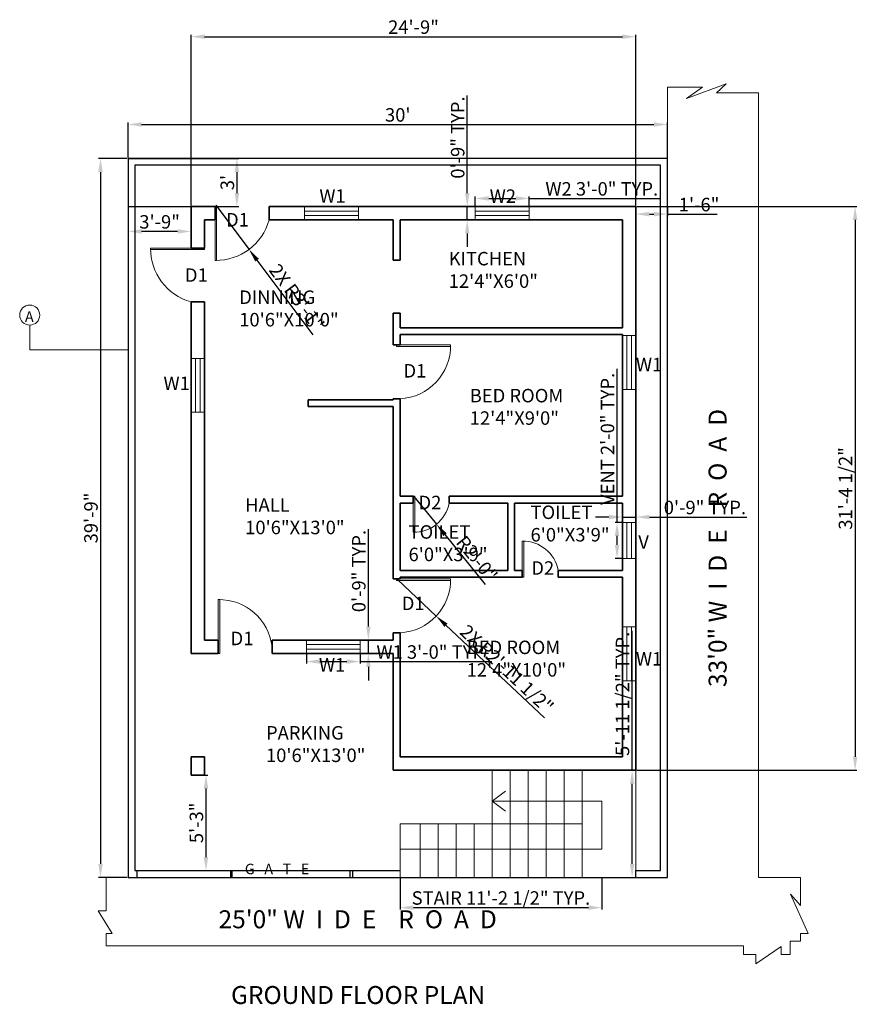
# Model space of a CAD drawing. Units: inches. Extents: x 2044 to 3644, y 808 to 1988.
# Tile 1 of 4: x 2044 to 2610, y 808 to 1466. Entities that reach past the tile are written whole.
import ezdxf

# ---------------------------------------------------------------- set-up
doc = ezdxf.new("R2010")
doc.units = ezdxf.units.IN
for name, color, linetype, lineweight in [('A-ANNO-DIMS', 2, 'Continuous', 18), ('A-ANNO-SYMB', 2, 'Continuous', 18), ('A-ANNO-TEXT', 7, 'Continuous', 18), ('A-ANNO-TITL', 7, 'Continuous', 25), ('A-AREA-IDEN', 7, 'Continuous', 18), ('A-COLS', 1, 'Continuous', 35), ('A-DOOR', 4, 'Continuous', 18), ('A-FLOR-STRS', 3, 'Continuous', 18), ('A-GLAZ', 4, 'Continuous', 18), ('A-WALL', 7, 'Continuous', 35), ('C-PROP', 3, 'Continuous', 25), ('C-ROAD', 8, 'Continuous', 18)]:
    doc.layers.add(name, color=color, linetype=linetype, lineweight=lineweight)
doc.styles.get("Standard").update_dxf_attribs({"font": 'arial.ttf'})
doc.dimstyles.new('ISO-25', dxfattribs={"dimtxt": 9, "dimasz": 9, "dimexe": 1.25, "dimexo": 0.625, "dimtad": 1, "dimdec": 1, "dimrnd": 9, "dimlunit": 3, "dimtxsty": 'Standard', "dimcen": 2.5, "dimadec": 0, "dimazin": 0, "dimtfac": 1, "dimtdec": 1, "dimtmove": 0, "dimatfit": 3, "dimfxl": 1, "dimarcsym": 0})

# ---------------------------------------------------------------- blocks, each defined once
blk = doc.blocks.new('*D1')
at = {"layer": 'A-ANNO-DIMS', "color": 0, "lineweight": -2, "transparency": 16777216}
for p, q in [((2455.33, 1340.62), (2455.33, 1334.91)), ((2464.33, 1336.16), (2467.33, 1336.16)), ((2476.33, 1340.62), (2476.33, 1334.91)), ((2476.33, 1336.16), (2509.65, 1336.16))]:
    blk.add_line(p, q, dxfattribs=at)
at = {"layer": 'A-ANNO-DIMS', "color": 0, "transparency": 16777216}
for points in [[(2464.33, 1337.66), (2464.33, 1334.66), (2455.33, 1336.16)], [(2467.33, 1337.66), (2467.33, 1334.66), (2476.33, 1336.16)]]:
    blk.add_solid(points, dxfattribs=at)
at = {"layer": 'Defpoints', "color": 0, "transparency": 16777216}
for p in [(2455.33, 1341.25), (2476.33, 1341.25), (2476.33, 1336.16)]:
    blk.add_point(p, dxfattribs=at)
at = {"layer": 'A-ANNO-DIMS', "color": 0, "transparency": 16777216, "insert": (2497.49, 1341.38), "char_height": 9, "attachment_point": 5}
blk.add_mtext('1\'-6"', dxfattribs=at)
blk = doc.blocks.new('*D2')
at = {"layer": 'A-ANNO-DIMS', "color": 0, "lineweight": -2, "transparency": 16777216}
for p, q in [((2116.95, 1373.25), (2190.19, 1373.25)), ((2188.94, 1364.25), (2188.94, 1350.25)), ((2116.95, 1341.25), (2190.19, 1341.25))]:
    blk.add_line(p, q, dxfattribs=at)
at = {"layer": 'A-ANNO-DIMS', "color": 0, "transparency": 16777216}
for points in [[(2187.44, 1364.25), (2190.44, 1364.25), (2188.94, 1373.25)], [(2187.44, 1350.25), (2190.44, 1350.25), (2188.94, 1341.25)]]:
    blk.add_solid(points, dxfattribs=at)
at = {"layer": 'Defpoints', "color": 0, "transparency": 16777216}
for p in [(2116.33, 1373.25), (2116.33, 1341.25), (2188.94, 1341.25)]:
    blk.add_point(p, dxfattribs=at)
at = {"layer": 'A-ANNO-DIMS', "color": 0, "transparency": 16777216, "insert": (2183.71, 1357.25), "char_height": 9, "attachment_point": 5, "rotation": 90}
blk.add_mtext("3'", dxfattribs=at)
blk = doc.blocks.new('*D3')
at = {"layer": 'A-ANNO-DIMS', "color": 0, "lineweight": -2, "transparency": 16777216}
for p, q in [((2116.33, 1340.62), (2116.33, 1323.36)), ((2158.33, 1340.62), (2158.33, 1323.36)), ((2149.33, 1324.61), (2125.33, 1324.61))]:
    blk.add_line(p, q, dxfattribs=at)
at = {"layer": 'A-ANNO-DIMS', "color": 0, "transparency": 16777216}
for points in [[(2125.33, 1326.11), (2125.33, 1323.11), (2116.33, 1324.61)], [(2149.33, 1326.11), (2149.33, 1323.11), (2158.33, 1324.61)]]:
    blk.add_solid(points, dxfattribs=at)
at = {"layer": 'Defpoints', "color": 0, "transparency": 16777216}
for p in [(2116.33, 1341.25), (2158.33, 1341.25), (2116.33, 1324.61)]:
    blk.add_point(p, dxfattribs=at)
at = {"layer": 'A-ANNO-DIMS', "color": 0, "transparency": 16777216, "insert": (2137.33, 1329.83), "char_height": 9, "width": 23.9181, "attachment_point": 5}
blk.add_mtext('3\'-9"', dxfattribs=at)
blk = doc.blocks.new('*D4')
at = {"layer": 'A-ANNO-DIMS', "color": 0, "lineweight": -2, "transparency": 16777216}
for p, q in [((2116.33, 1373.87), (2116.33, 1397.29)), ((2125.33, 1396.04), (2467.33, 1396.04)), ((2476.33, 1373.87), (2476.33, 1397.29))]:
    blk.add_line(p, q, dxfattribs=at)
at = {"layer": 'A-ANNO-DIMS', "color": 0, "transparency": 16777216}
for points in [[(2125.33, 1397.54), (2125.33, 1394.54), (2116.33, 1396.04)], [(2467.33, 1397.54), (2467.33, 1394.54), (2476.33, 1396.04)]]:
    blk.add_solid(points, dxfattribs=at)
at = {"layer": 'Defpoints', "color": 0, "transparency": 16777216}
for p in [(2476.33, 1396.04), (2116.33, 1373.25), (2476.33, 1373.25)]:
    blk.add_point(p, dxfattribs=at)
at = {"layer": 'A-ANNO-DIMS', "color": 0, "transparency": 16777216, "insert": (2296.33, 1401.26), "char_height": 9, "attachment_point": 5}
blk.add_mtext("30'", dxfattribs=at)
blk = doc.blocks.new('*D5')
at = {"layer": 'A-ANNO-DIMS', "color": 0, "lineweight": -2, "transparency": 16777216}
for p, q in [((2115.7, 1373.25), (2096.63, 1373.25)), ((2097.88, 1364.25), (2097.88, 902.25)), ((2115.7, 893.25), (2096.63, 893.25))]:
    blk.add_line(p, q, dxfattribs=at)
at = {"layer": 'A-ANNO-DIMS', "color": 0, "transparency": 16777216}
for points in [[(2096.38, 1364.25), (2099.38, 1364.25), (2097.88, 1373.25)], [(2096.38, 902.25), (2099.38, 902.25), (2097.88, 893.25)]]:
    blk.add_solid(points, dxfattribs=at)
at = {"layer": 'Defpoints', "color": 0, "transparency": 16777216}
for p in [(2116.33, 1373.25), (2097.88, 893.25), (2116.33, 893.25)]:
    blk.add_point(p, dxfattribs=at)
at = {"layer": 'A-ANNO-DIMS', "color": 0, "transparency": 16777216, "insert": (2092.66, 1133.25), "char_height": 9, "attachment_point": 5, "rotation": 90}
blk.add_mtext('39\'-9"', dxfattribs=at)
blk = doc.blocks.new('*D7')
at = {"layer": 'A-ANNO-DIMS', "color": 0, "lineweight": -2, "transparency": 16777216}
for p, q in [((2158.95, 961.56), (2169.53, 961.56)), ((2168.28, 952.56), (2168.28, 906.75)), ((2158.95, 897.75), (2169.53, 897.75))]:
    blk.add_line(p, q, dxfattribs=at)
at = {"layer": 'A-ANNO-DIMS', "color": 0, "transparency": 16777216}
for points in [[(2166.78, 952.56), (2169.78, 952.56), (2168.28, 961.56)], [(2166.78, 906.75), (2169.78, 906.75), (2168.28, 897.75)]]:
    blk.add_solid(points, dxfattribs=at)
at = {"layer": 'Defpoints', "color": 0, "transparency": 16777216}
for p in [(2158.33, 961.56), (2158.33, 897.75), (2168.28, 897.75)]:
    blk.add_point(p, dxfattribs=at)
at = {"layer": 'A-ANNO-DIMS', "color": 0, "transparency": 16777216, "insert": (2163.06, 929.65), "char_height": 9, "attachment_point": 5, "rotation": 90}
blk.add_mtext('5\'-3"', dxfattribs=at)
blk = doc.blocks.new('DOOR-D1-36-EXT')
for p, q in [((0, 36), (1, 36)), ((1, 36), (1, 0)), ((0, 0), (0, 27)), ((1, 0), (0, 0))]:
    blk.add_line(p, q)
blk.add_arc((0.5, 36.83), 36.84, 269.22228, 344.51752)
blk = doc.blocks.new('DOOR-D1-36-INT')
for p, q in [((0, 36), (0, 35)), ((0, 35), (36, 35)), ((36, 36), (2.25, 36)), ((36, 35), (36, 36))]:
    blk.add_line(p, q)
blk.add_arc((0.46, 35.5), 35.55, 272.88924, 0.80598)
blk = doc.blocks.new('DOOR-D2-24')
for p, q in [((0, 24), (1, 24)), ((1, 24), (1, 0)), ((0, 0), (0, 19.5)), ((1, 0), (0, 0))]:
    blk.add_line(p, q)
blk.add_arc((0.5, 23.9), 23.91, 268.80171, 349.38601)
blk = doc.blocks.new('WIN-W1-36')
for p, q in [((0, 9), (0, 0)), ((36, 9), (36, 0)), ((36, 6), (0, 6)), ((36, 3), (0, 3))]:
    blk.add_line(p, q)
blk = doc.blocks.new('WIN-W2-36')
for p, q in [((0, 9), (0, 0)), ((36, 9), (36, 0)), ((36, 6), (0, 6)), ((36, 3), (0, 3))]:
    blk.add_line(p, q)
blk = doc.blocks.new('VENT-24')
for p, q in [((0, 24), (9, 24)), ((3, 0), (3, 24)), ((6, 0), (6, 24)), ((0, 0), (9, 0))]:
    blk.add_line(p, q)
blk = doc.blocks.new('STAIR-RETURN-PLAN')
for p, q in [((61.5, 71.5), (61.5, 0)), ((73.5, 71.5), (73.5, 0)), ((85.5, 71.5), (85.5, 0)), ((97.5, 71.5), (97.5, 0)), ((109.5, 71.5), (109.5, 0)), ((121.5, 71.5), (121.5, 0)), ((61.5, 50.86), (70.45, 57.63)), ((134.75, 50.86), (61.5, 50.86)), ((61.5, 50.86), (70.45, 44.26)), ((134.75, 18.82), (134.75, 50.86)), ((0, 35.75), (0, 0)), ((121.5, 35.75), (0, 35.75)), ((13.5, 35.75), (13.5, 0)), ((25.5, 35.75), (25.5, 0)), ((37.5, 35.75), (37.5, 0)), ((49.5, 35.75), (49.5, 0)), ((0, 18.82), (134.75, 18.82))]:
    blk.add_line(p, q)
blk = doc.blocks.new('SECTION-MARK-ELBOW')
for p, q in [((6.87, 0), (6.87, 16.52)), ((72.41, 0), (6.87, 0))]:
    blk.add_line(p, q)
blk.add_circle((6.7, 23.26), 6.7)
blk = doc.blocks.new('*D29')
at = {"layer": 'A-ANNO-DIMS', "color": 0, "lineweight": -2, "transparency": 16777216}
for p, q in [((2235.3, 1042.12), (2235.3, 1036.1)), ((2271.3, 1042.12), (2271.3, 1036.1)), ((2244.3, 1037.35), (2262.3, 1037.35)), ((2271.3, 1037.35), (2359.13, 1037.35))]:
    blk.add_line(p, q, dxfattribs=at)
at = {"layer": 'A-ANNO-DIMS', "color": 0, "transparency": 16777216}
for points in [[(2244.3, 1038.85), (2244.3, 1035.85), (2235.3, 1037.35)], [(2262.3, 1038.85), (2262.3, 1035.85), (2271.3, 1037.35)]]:
    blk.add_solid(points, dxfattribs=at)
at = {"layer": 'Defpoints', "color": 0, "transparency": 16777216}
for p in [(2235.3, 1042.75), (2271.3, 1042.75), (2271.3, 1037.35)]:
    blk.add_point(p, dxfattribs=at)
at = {"layer": 'A-ANNO-DIMS', "color": 0, "transparency": 16777216, "insert": (2319.71, 1042.57), "char_height": 9, "attachment_point": 5}
blk.add_mtext('W1 3\'-0" TYP.', dxfattribs=at)
blk = doc.blocks.new('*D30')
at = {"layer": 'A-ANNO-DIMS', "color": 0, "lineweight": -2, "transparency": 16777216}
for p, q in [((2276.7, 1060.75), (2276.7, 1125.86)), ((2271.92, 1051.75), (2277.95, 1051.75)), ((2276.7, 1042.75), (2276.7, 1051.75)), ((2271.92, 1042.75), (2277.95, 1042.75)), ((2276.7, 1033.75), (2276.7, 1024.75))]:
    blk.add_line(p, q, dxfattribs=at)
at = {"layer": 'A-ANNO-DIMS', "color": 0, "transparency": 16777216}
for points in [[(2275.2, 1060.75), (2278.2, 1060.75), (2276.7, 1051.75)], [(2275.2, 1033.75), (2278.2, 1033.75), (2276.7, 1042.75)]]:
    blk.add_solid(points, dxfattribs=at)
at = {"layer": 'Defpoints', "color": 0, "transparency": 16777216}
for p in [(2271.3, 1051.75), (2276.7, 1051.75), (2271.3, 1042.75)]:
    blk.add_point(p, dxfattribs=at)
at = {"layer": 'A-ANNO-DIMS', "color": 0, "transparency": 16777216, "insert": (2271.48, 1097.8), "char_height": 9, "attachment_point": 5, "rotation": 90}
blk.add_mtext('0\'-9" TYP.', dxfattribs=at)
blk = doc.blocks.new('*D31')
at = {"layer": 'A-ANNO-DIMS', "color": 0, "lineweight": -2, "transparency": 16777216}
for p, q in [((2348.11, 1341.87), (2348.11, 1347.9)), ((2357.11, 1346.65), (2375.11, 1346.65)), ((2384.11, 1341.87), (2384.11, 1347.9)), ((2384.11, 1346.65), (2471.94, 1346.65))]:
    blk.add_line(p, q, dxfattribs=at)
at = {"layer": 'A-ANNO-DIMS', "color": 0, "transparency": 16777216}
for points in [[(2357.11, 1348.15), (2357.11, 1345.15), (2348.11, 1346.65)], [(2375.11, 1348.15), (2375.11, 1345.15), (2384.11, 1346.65)]]:
    blk.add_solid(points, dxfattribs=at)
at = {"layer": 'Defpoints', "color": 0, "transparency": 16777216}
for p in [(2384.11, 1346.65), (2348.11, 1341.25), (2384.11, 1341.25)]:
    blk.add_point(p, dxfattribs=at)
at = {"layer": 'A-ANNO-DIMS', "color": 0, "transparency": 16777216, "insert": (2432.53, 1351.87), "char_height": 9, "attachment_point": 5}
blk.add_mtext('W2 3\'-0" TYP.', dxfattribs=at)
blk = doc.blocks.new('*D32')
at = {"layer": 'A-ANNO-DIMS', "color": 0, "lineweight": -2, "transparency": 16777216}
for p, q in [((2342.71, 1350.25), (2342.71, 1415.36)), ((2347.49, 1341.25), (2341.46, 1341.25)), ((2342.71, 1332.25), (2342.71, 1341.25)), ((2347.49, 1332.25), (2341.46, 1332.25)), ((2342.71, 1323.25), (2342.71, 1314.25))]:
    blk.add_line(p, q, dxfattribs=at)
at = {"layer": 'A-ANNO-DIMS', "color": 0, "transparency": 16777216}
for points in [[(2341.21, 1350.25), (2344.21, 1350.25), (2342.71, 1341.25)], [(2341.21, 1323.25), (2344.21, 1323.25), (2342.71, 1332.25)]]:
    blk.add_solid(points, dxfattribs=at)
at = {"layer": 'Defpoints', "color": 0, "transparency": 16777216}
for p in [(2342.71, 1341.25), (2348.11, 1341.25), (2348.11, 1332.25)]:
    blk.add_point(p, dxfattribs=at)
at = {"layer": 'A-ANNO-DIMS', "color": 0, "transparency": 16777216, "insert": (2337.49, 1387.3), "char_height": 9, "attachment_point": 5, "rotation": 90}
blk.add_mtext('0\'-9" TYP.', dxfattribs=at)
blk = doc.blocks.new('*D39')
at = {"layer": 'A-ANNO-DIMS', "color": 0, "lineweight": -2, "transparency": 16777216}
for p, q in [((2442.73, 1130.26), (2442.73, 1232.86)), ((2445.7, 1130.26), (2441.48, 1130.26)), ((2442.73, 1115.26), (2442.73, 1121.26)), ((2445.7, 1106.26), (2441.48, 1106.26))]:
    blk.add_line(p, q, dxfattribs=at)
at = {"layer": 'A-ANNO-DIMS', "color": 0, "transparency": 16777216}
for points in [[(2441.23, 1121.26), (2444.23, 1121.26), (2442.73, 1130.26)], [(2441.23, 1115.26), (2444.23, 1115.26), (2442.73, 1106.26)]]:
    blk.add_solid(points, dxfattribs=at)
at = {"layer": 'Defpoints', "color": 0, "transparency": 16777216}
for p in [(2442.73, 1130.26), (2446.33, 1130.26), (2446.33, 1106.26)]:
    blk.add_point(p, dxfattribs=at)
at = {"layer": 'A-ANNO-DIMS', "color": 0, "transparency": 16777216, "insert": (2437.51, 1186.06), "char_height": 9, "attachment_point": 5, "rotation": 90}
blk.add_mtext('VENT 2\'-0" TYP.', dxfattribs=at)
blk = doc.blocks.new('*D40')
at = {"layer": 'A-ANNO-DIMS', "color": 0, "lineweight": -2, "transparency": 16777216}
for p, q in [((2437.33, 1133.86), (2428.33, 1133.86)), ((2446.33, 1130.88), (2446.33, 1135.11)), ((2446.33, 1133.86), (2455.33, 1133.86)), ((2455.33, 1130.88), (2455.33, 1135.11)), ((2464.33, 1133.86), (2529.44, 1133.86))]:
    blk.add_line(p, q, dxfattribs=at)
at = {"layer": 'A-ANNO-DIMS', "color": 0, "transparency": 16777216}
for points in [[(2437.33, 1135.36), (2437.33, 1132.36), (2446.33, 1133.86)], [(2464.33, 1135.36), (2464.33, 1132.36), (2455.33, 1133.86)]]:
    blk.add_solid(points, dxfattribs=at)
at = {"layer": 'Defpoints', "color": 0, "transparency": 16777216}
for p in [(2455.33, 1133.86), (2446.33, 1130.26), (2455.33, 1130.26)]:
    blk.add_point(p, dxfattribs=at)
at = {"layer": 'A-ANNO-DIMS', "color": 0, "transparency": 16777216, "insert": (2501.38, 1139.08), "char_height": 9, "attachment_point": 5}
blk.add_mtext('0\'-9" TYP.', dxfattribs=at)
blk = doc.blocks.new('*D41')
at = {"layer": 'A-ANNO-DIMS', "color": 0, "lineweight": -2, "transparency": 16777216}
for p, q in [((2297.83, 892.62), (2297.83, 871.79)), ((2432.57, 892.62), (2432.57, 871.79)), ((2306.83, 873.04), (2423.57, 873.04))]:
    blk.add_line(p, q, dxfattribs=at)
at = {"layer": 'A-ANNO-DIMS', "color": 0, "transparency": 16777216}
for points in [[(2306.83, 874.54), (2306.83, 871.54), (2297.83, 873.04)], [(2423.57, 874.54), (2423.57, 871.54), (2432.57, 873.04)]]:
    blk.add_solid(points, dxfattribs=at)
at = {"layer": 'Defpoints', "color": 0, "transparency": 16777216}
for p in [(2297.83, 893.25), (2432.57, 893.25), (2432.57, 873.04)]:
    blk.add_point(p, dxfattribs=at)
at = {"layer": 'A-ANNO-DIMS', "color": 0, "transparency": 16777216, "insert": (2365.2, 878.31), "char_height": 9, "attachment_point": 5}
blk.add_mtext('STAIR 11\'-2 1/2" TYP.', dxfattribs=at)
blk = doc.blocks.new('*D42')
at = {"layer": 'A-ANNO-DIMS', "color": 0, "lineweight": -2, "transparency": 16777216}
for p, q in [((2452.79, 964.75), (2452.79, 1057.82)), ((2433.2, 964.75), (2454.04, 964.75)), ((2452.79, 902.25), (2452.79, 955.75)), ((2433.2, 893.25), (2454.04, 893.25))]:
    blk.add_line(p, q, dxfattribs=at)
at = {"layer": 'A-ANNO-DIMS', "color": 0, "transparency": 16777216}
for points in [[(2451.29, 955.75), (2454.29, 955.75), (2452.79, 964.75)], [(2451.29, 902.25), (2454.29, 902.25), (2452.79, 893.25)]]:
    blk.add_solid(points, dxfattribs=at)
at = {"layer": 'Defpoints', "color": 0, "transparency": 16777216}
for p in [(2432.57, 964.75), (2452.79, 964.75), (2432.57, 893.25)]:
    blk.add_point(p, dxfattribs=at)
at = {"layer": 'A-ANNO-DIMS', "color": 0, "transparency": 16777216, "insert": (2447.51, 1015.78), "char_height": 9, "attachment_point": 5, "rotation": 90}
blk.add_mtext('5\'-11 1/2" TYP.', dxfattribs=at)
blk = doc.blocks.new('*D51')
at = {"layer": 'A-ANNO-DIMS', "color": 0, "lineweight": -2, "transparency": 16777216}
for p, q in [((2158.33, 1341.87), (2158.33, 1455.91)), ((2167.33, 1454.66), (2446.33, 1454.66)), ((2455.33, 1341.87), (2455.33, 1455.91))]:
    blk.add_line(p, q, dxfattribs=at)
at = {"layer": 'A-ANNO-DIMS', "color": 0, "transparency": 16777216}
for points in [[(2167.33, 1456.16), (2167.33, 1453.16), (2158.33, 1454.66)], [(2446.33, 1456.16), (2446.33, 1453.16), (2455.33, 1454.66)]]:
    blk.add_solid(points, dxfattribs=at)
at = {"layer": 'Defpoints', "color": 0, "transparency": 16777216}
for p in [(2455.33, 1454.66), (2158.33, 1341.25), (2455.33, 1341.25)]:
    blk.add_point(p, dxfattribs=at)
at = {"layer": 'A-ANNO-DIMS', "color": 0, "transparency": 16777216, "insert": (2306.83, 1459.88), "char_height": 9, "attachment_point": 5}
blk.add_mtext('24\'-9"', dxfattribs=at)
blk = doc.blocks.new('*D52')
at = {"layer": 'A-ANNO-DIMS', "color": 0, "lineweight": -2, "transparency": 16777216}
for p, q in [((2455.95, 1341.25), (2602.92, 1341.25)), ((2601.67, 1332.25), (2601.67, 973.75)), ((2455.95, 964.75), (2602.92, 964.75))]:
    blk.add_line(p, q, dxfattribs=at)
at = {"layer": 'A-ANNO-DIMS', "color": 0, "transparency": 16777216}
for points in [[(2600.17, 1332.25), (2603.17, 1332.25), (2601.67, 1341.25)], [(2600.17, 973.75), (2603.17, 973.75), (2601.67, 964.75)]]:
    blk.add_solid(points, dxfattribs=at)
at = {"layer": 'Defpoints', "color": 0, "transparency": 16777216}
for p in [(2455.33, 1341.25), (2455.33, 964.75), (2601.67, 964.75)]:
    blk.add_point(p, dxfattribs=at)
at = {"layer": 'A-ANNO-DIMS', "color": 0, "transparency": 16777216, "insert": (2596.39, 1153), "char_height": 9, "attachment_point": 5, "rotation": 90}
blk.add_mtext('31\'-4 1/2"', dxfattribs=at)
blk = doc.blocks.new('*D76')
at = {"layer": 'A-ANNO-DIMS', "color": 0, "lineweight": -2, "transparency": 16777216}
for p, q in [((2174.91, 1342.08), (2197.01, 1312.61)), ((2239.77, 1255.59), (2202.41, 1305.41))]:
    blk.add_line(p, q, dxfattribs=at)
at = {"layer": 'A-ANNO-DIMS', "color": 0, "transparency": 16777216}
blk.add_solid([(2203.61, 1306.31), (2201.21, 1304.51), (2197.01, 1312.61)], dxfattribs=at)
at = {"layer": 'Defpoints', "color": 0, "transparency": 16777216}
for p in [(2174.91, 1342.08), (2197.01, 1312.61)]:
    blk.add_point(p, dxfattribs=at)
at = {"layer": 'A-ANNO-DIMS', "color": 0, "transparency": 16777216, "insert": (2227.97, 1280.03), "char_height": 9, "attachment_point": 5, "rotation": 306.86988}
blk.add_mtext('2X R3\'-1"', dxfattribs=at)
blk = doc.blocks.new('*D78')
at = {"layer": 'A-ANNO-DIMS', "color": 0, "lineweight": -2, "transparency": 16777216}
for p, q in [((2296.04, 1092.07), (2321.97, 1067.76)), ((2394.37, 999.89), (2328.53, 1061.61))]:
    blk.add_line(p, q, dxfattribs=at)
at = {"layer": 'A-ANNO-DIMS', "color": 0, "transparency": 16777216}
blk.add_solid([(2329.56, 1062.7), (2327.51, 1060.51), (2321.97, 1067.76)], dxfattribs=at)
at = {"layer": 'Defpoints', "color": 0, "transparency": 16777216}
for p in [(2296.04, 1092.07), (2321.97, 1067.76)]:
    blk.add_point(p, dxfattribs=at)
at = {"layer": 'A-ANNO-DIMS', "color": 0, "transparency": 16777216, "insert": (2368.34, 1031.52), "char_height": 9, "attachment_point": 5, "rotation": 316.8468}
blk.add_mtext('2X R2\'-11 1/2"', dxfattribs=at)
blk = doc.blocks.new('*D79')
at = {"layer": 'A-ANNO-DIMS', "color": 0, "lineweight": -2, "transparency": 16777216}
for p, q in [((2307.12, 1147.65), (2322.19, 1129.1)), ((2354.85, 1088.9), (2327.87, 1122.11))]:
    blk.add_line(p, q, dxfattribs=at)
at = {"layer": 'A-ANNO-DIMS', "color": 0, "transparency": 16777216}
blk.add_solid([(2329.03, 1123.06), (2326.71, 1121.16), (2322.19, 1129.1)], dxfattribs=at)
at = {"layer": 'Defpoints', "color": 0, "transparency": 16777216}
for p in [(2307.12, 1147.65), (2322.19, 1129.1)]:
    blk.add_point(p, dxfattribs=at)
at = {"layer": 'A-ANNO-DIMS', "color": 0, "transparency": 16777216, "insert": (2348.25, 1105.31), "char_height": 9, "attachment_point": 5, "rotation": 309.09468}
blk.add_mtext('R2\'-0"', dxfattribs=at)

msp = doc.modelspace()

# ---------------------------------------------------------------- linework, layer by layer
at = {"layer": 'A-COLS'}
for p, q in [((2158.33, 973.75), (2167.33, 973.75)), ((2158.33, 961.56), (2158.33, 973.75)), ((2167.33, 973.75), (2167.33, 961.56)), ((2167.33, 961.56), (2158.33, 961.56))]:
    msp.add_line(p, q, dxfattribs=at)
at = {"layer": 'A-DOOR'}
for p, q in [((2177.45, 1078.75), (2176.45, 1078.75)), ((2176.45, 1078.75), (2176.45, 1051.75)), ((2177.45, 1042.75), (2177.45, 1078.75)), ((2176.45, 1042.75), (2177.45, 1042.75))]:
    msp.add_line(p, q, dxfattribs=at)
msp.add_arc((2176.95, 1043), 35.75, 6.82686, 90.80129, dxfattribs=at)
at = {"layer": 'A-FLOR-STRS'}
msp.add_line((2455.33, 964.75), (2455.33, 893.25), dxfattribs=at)
at = {"layer": 'A-WALL'}
for p, q in [((2158.33, 1341.25), (2158.33, 1313.53)), ((2174.41, 1341.25), (2158.33, 1341.25)), ((2174.41, 1341.25), (2174.41, 1332.25)), ((2455.33, 1341.25), (2210.41, 1341.25)), ((2210.41, 1341.25), (2210.41, 1332.25)), ((2455.33, 964.75), (2455.33, 1341.25)), ((2167.33, 1332.25), (2167.33, 1313.53)), ((2174.41, 1332.25), (2167.33, 1332.25)), ((2293.33, 1332.25), (2210.41, 1332.25)), ((2293.33, 1332.25), (2293.33, 1305.52)), ((2446.33, 1332.25), (2297.83, 1332.25)), ((2297.83, 1332.25), (2297.83, 1305.52)), ((2446.33, 1260.25), (2446.33, 1332.25)), ((2167.33, 1313.53), (2158.33, 1313.53)), ((2297.83, 1305.52), (2293.33, 1305.52)), ((2167.33, 1277.53), (2158.33, 1277.53)), ((2158.33, 1277.53), (2158.33, 1042.75)), ((2167.33, 1277.53), (2167.33, 1212.25)), ((2297.83, 1269.95), (2293.33, 1269.95)), ((2293.33, 1269.95), (2293.33, 1248.85)), ((2297.83, 1269.95), (2297.83, 1260.25)), ((2446.33, 1260.25), (2297.83, 1260.25)), ((2446.33, 1255.75), (2297.83, 1255.75)), ((2297.83, 1255.75), (2297.83, 1248.85)), ((2446.33, 1147.75), (2446.33, 1255.75)), ((2297.83, 1248.85), (2293.33, 1248.85)), ((2167.33, 1212.25), (2167.33, 1207.75)), ((2293.33, 1212.25), (2236.44, 1212.25)), ((2236.44, 1212.25), (2236.44, 1207.75)), ((2297.83, 1212.85), (2293.33, 1212.85)), ((2293.33, 1212.85), (2293.33, 1212.25)), ((2297.83, 1212.85), (2297.83, 1147.75)), ((2167.33, 1207.75), (2167.33, 1051.75)), ((2293.33, 1207.75), (2236.44, 1207.75)), ((2293.33, 1207.75), (2293.33, 1092.57)), ((2306.62, 1147.75), (2297.83, 1147.75)), ((2306.62, 1147.75), (2306.62, 1143.25)), ((2446.33, 1147.75), (2330.62, 1147.75)), ((2330.62, 1147.75), (2330.62, 1143.25)), ((2297.83, 1143.25), (2297.83, 1098.25)), ((2306.62, 1143.25), (2297.83, 1143.25)), ((2369.83, 1143.25), (2330.62, 1143.25)), ((2369.83, 1098.25), (2369.83, 1143.25)), ((2446.33, 1143.25), (2374.33, 1143.25)), ((2374.33, 1098.25), (2374.33, 1143.25)), ((2446.33, 1098.25), (2446.33, 1143.25)), ((2369.83, 1098.25), (2297.83, 1098.25)), ((2379.43, 1098.25), (2374.33, 1098.25)), ((2379.43, 1098.25), (2379.43, 1093.75)), ((2446.33, 1098.25), (2403.43, 1098.25)), ((2403.43, 1098.25), (2403.43, 1093.75)), ((2297.83, 1092.57), (2293.33, 1092.57)), ((2297.83, 1093.75), (2297.83, 1092.57)), ((2379.43, 1093.75), (2297.83, 1093.75)), ((2446.33, 1093.75), (2403.43, 1093.75)), ((2446.33, 973.75), (2446.33, 1093.75)), ((2297.83, 1056.57), (2293.33, 1056.57)), ((2293.33, 1056.57), (2293.33, 1051.75)), ((2297.83, 1056.57), (2297.83, 973.75)), ((2176.45, 1051.75), (2167.33, 1051.75)), ((2176.45, 1051.75), (2176.45, 1042.75)), ((2293.33, 1051.75), (2212.45, 1051.75)), ((2212.45, 1051.75), (2212.45, 1042.75)), ((2176.45, 1042.75), (2158.33, 1042.75)), ((2293.33, 1042.75), (2212.45, 1042.75)), ((2293.33, 1042.75), (2293.33, 964.75)), ((2446.33, 973.75), (2297.83, 973.75)), ((2455.33, 964.75), (2293.33, 964.75))]:
    msp.add_line(p, q, dxfattribs=at)
at = {"layer": 'C-PROP'}
for p, q in [((2476.33, 1373.25), (2116.33, 1373.25)), ((2116.33, 1373.25), (2116.33, 893.25)), ((2471.83, 1368.75), (2120.83, 1368.75)), ((2120.83, 1368.75), (2120.83, 897.75)), ((2471.83, 897.75), (2471.83, 1368.75)), ((2476.33, 893.25), (2476.33, 1373.25)), ((2120.83, 897.75), (2297.83, 897.75)), ((2122.2, 897.75), (2122.2, 893.25)), ((2184.73, 897.75), (2184.73, 893.25)), ((2185.45, 897.75), (2185.45, 893.25)), ((2264.36, 897.75), (2264.36, 893.25)), ((2266.09, 897.75), (2266.09, 893.25)), ((2455.33, 893.25), (2455.33, 897.75)), ((2455.33, 897.75), (2471.83, 897.75)), ((2116.33, 893.25), (2476.33, 893.25))]:
    msp.add_line(p, q, dxfattribs=at)
at = {"layer": 'C-ROAD'}
for p, q in [((2476.33, 1373.25), (2476.33, 1420.95)), ((2476.33, 1420.95), (2499.86, 1420.95)), ((2489.13, 1413.45), (2515.56, 1423.26)), ((2499.86, 1420.95), (2489.13, 1413.45)), ((2515.56, 1423.26), (2509.14, 1417.22)), ((2509.14, 1417.22), (2537.08, 1417.22)), ((2537.08, 1417.22), (2537.08, 893.25)), ((2101.63, 870.94), (2101.63, 893.25)), ((2537.08, 893.25), (2565.3, 893.25)), ((2565.3, 893.25), (2565.3, 874.47)), ((2565.3, 874.47), (2558.51, 881.98)), ((2558.51, 881.98), (2570.27, 855.84)), ((2105.62, 855.72), (2096.29, 870.94)), ((2096.29, 870.94), (2101.63, 870.94)), ((2101.63, 847.46), (2101.63, 855.72)), ((2101.63, 855.72), (2105.62, 855.72)), ((2570.27, 855.84), (2565.3, 855.84)), ((2565.3, 855.84), (2565.3, 850.65)), ((2565.3, 850.65), (2558.38, 850.65)), ((2558.38, 850.65), (2558.38, 841.67)), ((2527.2, 847.46), (2101.63, 847.46)), ((2527.2, 841.77), (2527.2, 847.46)), ((2535.39, 841.77), (2527.2, 841.77)), ((2552.29, 847.16), (2535.39, 835.6)), ((2535.39, 835.6), (2535.39, 841.77)), ((2552.29, 841.67), (2552.29, 847.16)), ((2558.38, 841.67), (2552.29, 841.67))]:
    msp.add_line(p, q, dxfattribs=at)

# ---------------------------------------------------------------- block references
at = {"layer": 'A-ANNO-SYMB'}
msp.add_blockref('SECTION-MARK-ELBOW', (2043.92, 1245.5), dxfattribs=at)
at = {"layer": 'A-DOOR'}
for name, p in [('DOOR-D1-36-EXT', (2174.41, 1305.25)), ('DOOR-D1-36-INT', (2295.58, 1212.85)), ('DOOR-D2-24', (2306.62, 1123.75)), ('DOOR-D1-36-INT', (2295.58, 1056.57))]:
    msp.add_blockref(name, p, dxfattribs=at)
at = {"layer": 'A-DOOR', "rotation": 270.0000000000001}
msp.add_blockref('DOOR-D1-36-EXT', (2131.33, 1313.53), dxfattribs=at)
at = {"layer": 'A-DOOR', "extrusion": (0, 0, -1), "zscale": -1, "rotation": 180}
msp.add_blockref('DOOR-D2-24', (-2379.43, 1117.75), dxfattribs=at)
at = {"layer": 'A-FLOR-STRS'}
msp.add_blockref('STAIR-RETURN-PLAN', (2297.83, 893.25), dxfattribs=at)
at = {"layer": 'A-GLAZ'}
for name, p in [('WIN-W1-36', (2234.17, 1332.25)), ('WIN-W2-36', (2348.11, 1332.25)), ('VENT-24', (2446.33, 1106.26)), ('WIN-W1-36', (2235.3, 1042.75))]:
    msp.add_blockref(name, p, dxfattribs=at)
for p, rotation in [((2455.33, 1219.03), 90.00000000000003), ((2167.33, 1203.86), 89.99999999999984), ((2455.33, 1024.48), 90.00000000000053)]:
    msp.add_blockref('WIN-W1-36', p, dxfattribs=dict(at, rotation=rotation))

# ---------------------------------------------------------------- texts
at = {"layer": 'A-ANNO-SYMB', "insert": (2047.44, 1271.23), "char_height": 7, "attachment_point": 1}
msp.add_mtext_dynamic_manual_height_columns('A', width=7.8302, gutter_width=12.5, heights=[0], dxfattribs=at)
at = {"layer": 'A-ANNO-TEXT', "attachment_point": 1}
for s, width, insert, char_height in [('W1', 19.1778, (2243.98, 1352.81), 9), ('W2', 19.1778, (2357.69, 1352.69), 9), ('D1', 19.1778, (2181.67, 1336.9), 9), ('D1', 19.1778, (2154.22, 1299.96), 9), ('W1', 19.1778, (2455.33, 1240.22), 9), ('D1', 19.1778, (2300.16, 1236.04), 9), ('W1', 19.1778, (2139.92, 1227.67), 9), ('D2', 19.1778, (2310.18, 1148.08), 9), ('V', 19.1778, (2456.91, 1121.67), 9), ('D2', 19.1778, (2385.5, 1104.34), 9), ('D1', 19.1778, (2299.01, 1080.73), 9), ('D1', 19.1778, (2184.71, 1057.29), 9), ('W1', 19.1778, (2243.72, 1039.66), 9), ('W1', 19.1778, (2455.33, 1043.69), 9), ('G   A   T   E', 81.5242, (2194.25, 902.36), 7), ('25\'0" W  I  D  E    R  O  A  D', 282.7276, (2176.68, 871.25), 12)]:
    msp.add_mtext_dynamic_manual_height_columns(s, width=width, gutter_width=12.5, heights=[0], dxfattribs=dict(at, insert=insert, char_height=char_height))
at = {"layer": 'A-ANNO-TEXT', "insert": (2503.87, 1020.31), "char_height": 12, "attachment_point": 1, "rotation": 90}
msp.add_mtext_dynamic_manual_height_columns('33\'0" W  I  D  E    R  O  A  D', width=282.7276, gutter_width=12.5, heights=[0], dxfattribs=at)
at = {"layer": 'A-ANNO-TITL', "insert": (2185.01, 820.68), "char_height": 12, "attachment_point": 1}
msp.add_mtext_dynamic_manual_height_columns('GROUND FLOOR PLAN', width=282.7276, gutter_width=12.5, heights=[0], dxfattribs=at)
at = {"layer": 'A-AREA-IDEN', "char_height": 9, "attachment_point": 1}
for s, insert in [('KITCHEN\\P12\'4"X6\'0"', (2330.33, 1310.93)), ('DINNING\\P10\'6"X10\'0"', (2190.48, 1285.17)), ('BED ROOM\\P12\'4"X9\'0"', (2344.37, 1219.46)), ('HALL\\P10\'6"X13\'0"', (2194.44, 1146.42)), ('TOILET\\P6\'0"X3\'9"', (2384.97, 1141.56)), ('TOILET\\P6\'0"X3\'9"', (2303.52, 1128.41)), ('BED ROOM\\P12\'4"X10\'0"', (2342.32, 1051.33)), ('PARKING\\P10\'6"X13\'0"', (2208.35, 994.27))]:
    msp.add_mtext_dynamic_manual_height_columns(s, width=86.1264, gutter_width=12.5, heights=[0], dxfattribs=dict(at, insert=insert))

# ---------------------------------------------------------------- dimensions: what is measured, and where the dimension line sits
at = {"layer": 'A-ANNO-DIMS'}
for base, p1, p2, override, picture, middle in [((2455.33, 1454.66), (2158.33, 1341.25), (2455.33, 1341.25), {"dimdec": 1, "dimlfac": 1, "dimrnd": 0, "dimzin": 1, "dimdsep": 46, "dimlunit": 4, "dimfrac": 2}, '*D51', (2306.83, 1459.88)), ((2476.33, 1396.04), (2116.33, 1373.25), (2476.33, 1373.25), {"dimclrd": 0, "dimclre": 0, "dimclrt": 0}, '*D4', (2296.33, 1401.26)), ((2476.33, 1336.16), (2455.33, 1341.25), (2476.33, 1341.25), {"dimclrd": 0, "dimclre": 0, "dimclrt": 0}, '*D1', (2497.49, 1341.38)), ((2116.33, 1324.61), (2158.33, 1341.25), (2116.33, 1341.25), {"dimclrd": 0, "dimclre": 0, "dimclrt": 0}, '*D3', (2137.33, 1329.83))]:
    dim = msp.add_linear_dim(base=base, p1=p1, p2=p2, dimstyle='ISO-25', override=override, dxfattribs=at)
    dim.commit()
    dim.dimension.update_dxf_attribs({"geometry": picture, "text_midpoint": middle})
for base, p1, p2, text, picture, middle in [((2342.71, 1341.25), (2348.11, 1332.25), (2348.11, 1341.25), '<> TYP.', '*D32', (2337.49, 1387.3)), ((2442.73, 1130.26), (2446.33, 1106.26), (2446.33, 1130.26), 'VENT <> TYP.', '*D39', (2437.51, 1186.06)), ((2276.7, 1051.75), (2271.3, 1042.75), (2271.3, 1051.75), '<> TYP.', '*D30', (2271.48, 1097.8)), ((2452.79, 964.75), (2432.57, 893.25), (2432.57, 964.75), '<> TYP.', '*D42', (2447.51, 1015.78))]:
    dim = msp.add_linear_dim(base=base, p1=p1, p2=p2, angle=90, text=text, dimstyle='ISO-25', override={"dimdec": 1, "dimlfac": 1, "dimrnd": 0, "dimzin": 1, "dimdsep": 46, "dimlunit": 4, "dimfrac": 2}, dxfattribs=at)
    dim.commit()
    dim.dimension.update_dxf_attribs({"geometry": picture, "text_midpoint": middle})
for base, p1, p2, override, picture, middle in [((2097.88, 893.25), (2116.33, 1373.25), (2116.33, 893.25), {"dimclrd": 0, "dimclre": 0, "dimclrt": 0}, '*D5', (2092.66, 1133.25)), ((2188.94, 1341.25), (2116.33, 1373.25), (2116.33, 1341.25), {"dimclrd": 0, "dimclre": 0, "dimclrt": 0}, '*D2', (2183.71, 1357.25)), ((2601.67, 964.75), (2455.33, 1341.25), (2455.33, 964.75), {"dimdec": 1, "dimlfac": 1, "dimrnd": 0, "dimzin": 1, "dimdsep": 46, "dimlunit": 4, "dimfrac": 2}, '*D52', (2596.39, 1153)), ((2168.28, 897.75), (2158.33, 961.56), (2158.33, 897.75), {"dimclrd": 0, "dimclre": 0, "dimclrt": 0}, '*D7', (2163.06, 929.65))]:
    dim = msp.add_linear_dim(base=base, p1=p1, p2=p2, angle=90, dimstyle='ISO-25', override=override, dxfattribs=at)
    dim.commit()
    dim.dimension.update_dxf_attribs({"geometry": picture, "text_midpoint": middle})
for base, p1, p2, text, picture, middle in [((2384.11, 1346.65), (2348.11, 1341.25), (2384.11, 1341.25), 'W2 <> TYP.', '*D31', (2432.53, 1351.87)), ((2455.33, 1133.86), (2446.33, 1130.26), (2455.33, 1130.26), '<> TYP.', '*D40', (2501.38, 1139.08)), ((2271.3, 1037.35), (2235.3, 1042.75), (2271.3, 1042.75), 'W1 <> TYP.', '*D29', (2319.71, 1042.57)), ((2432.57, 873.04), (2297.83, 893.25), (2432.57, 893.25), 'STAIR <> TYP.', '*D41', (2365.2, 878.31))]:
    dim = msp.add_linear_dim(base=base, p1=p1, p2=p2, text=text, dimstyle='ISO-25', override={"dimdec": 1, "dimlfac": 1, "dimrnd": 0, "dimzin": 1, "dimdsep": 46, "dimlunit": 4, "dimfrac": 2}, dxfattribs=at)
    dim.commit()
    dim.dimension.update_dxf_attribs({"geometry": picture, "text_midpoint": middle})
for center, mpoint, picture, middle in [((2174.91, 1342.08), (2197.01, 1312.61), '*D76', (2227.97, 1280.03)), ((2296.04, 1092.07), (2321.97, 1067.76), '*D78', (2368.34, 1031.52))]:
    dim = msp.add_radius_dim(center=center, mpoint=mpoint, text='2X <>', dimstyle='ISO-25', override={"dimdec": 1, "dimlfac": 1, "dimrnd": 0, "dimzin": 1, "dimdsep": 46, "dimlunit": 4, "dimfrac": 2}, dxfattribs=at)
    dim.commit()
    dim.dimension.update_dxf_attribs({"geometry": picture, "text_midpoint": middle})
dim = msp.add_radius_dim(center=(2307.12, 1147.65), mpoint=(2322.19, 1129.1), dimstyle='ISO-25', override={"dimdec": 1, "dimlfac": 1, "dimrnd": 0, "dimzin": 1, "dimdsep": 46, "dimlunit": 4, "dimfrac": 2}, dxfattribs=at)
dim.commit()
dim.dimension.update_dxf_attribs({"geometry": '*D79', "text_midpoint": (2348.25, 1105.31)})

doc.saveas('drawing.dxf')
